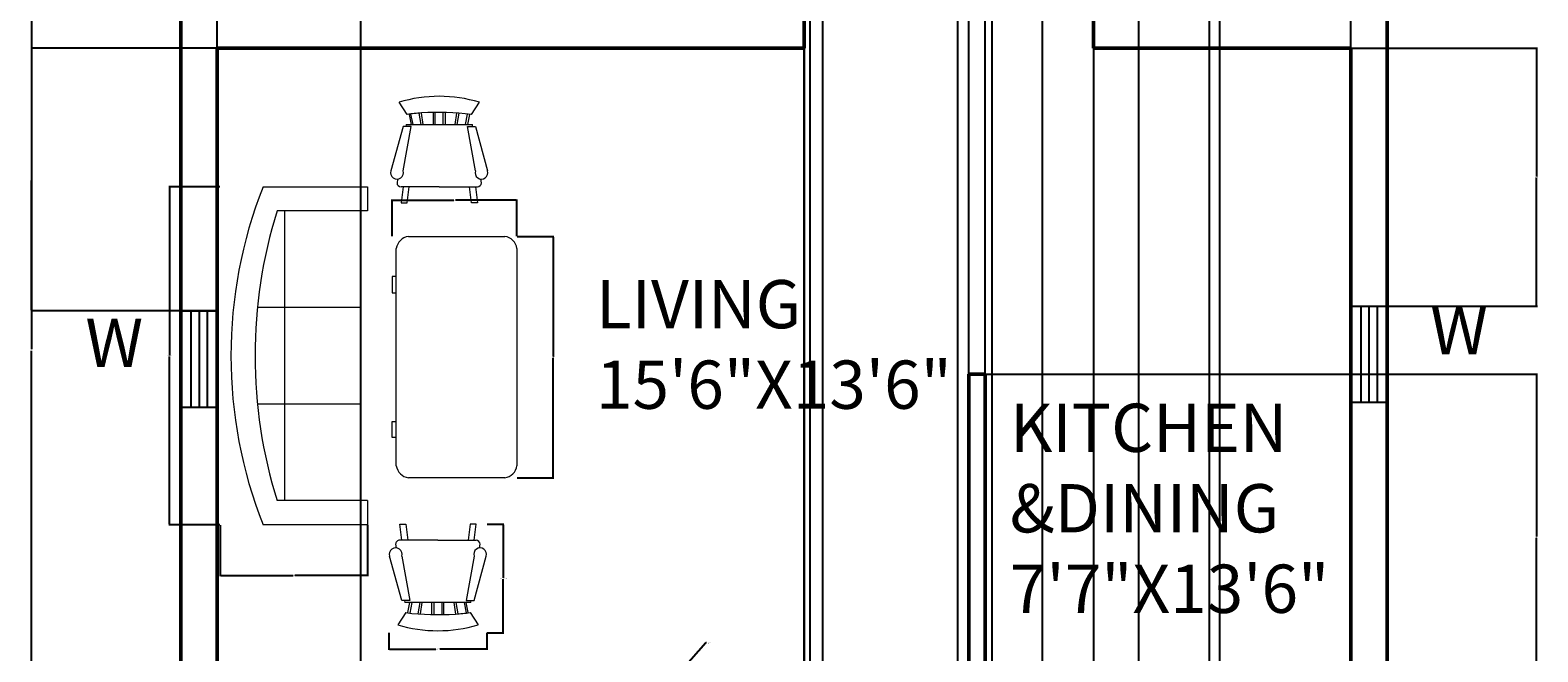
# Model space of a CAD drawing. Units: inches. Extents: x -15 to 361, y -684 to 58.
# Tile 2 of 3: x -15 to 360, y -385 to -230. Entities that reach past the tile are written whole.
import ezdxf

# ---------------------------------------------------------------- set-up
doc = ezdxf.new("R2010")
doc.units = ezdxf.units.IN
doc.header["$MEASUREMENT"] = 0
for name, color, linetype, lineweight in [('A-ANNO-DIMS', 2, 'Continuous', 18), ('A-ANNO-TEXT', 7, 'Continuous', 18), ('A-AREA-IDEN', 7, 'Continuous', 25), ('A-FURN', 8, 'Continuous', 18), ('A-GLAZ', 4, 'Continuous', 25), ('A-WALL', 7, 'Continuous', 50)]:
    doc.layers.add(name, color=color, linetype=linetype, lineweight=lineweight)
doc.styles.get("Standard").update_dxf_attribs({"font": 'arial.ttf'})
doc.dimstyles.get("Standard").update_dxf_attribs({"dimtxt": 0.18, "dimasz": 0.18, "dimexe": 0.18, "dimexo": 0.0625, "dimgap": 0.09, "dimtad": 0, "dimtih": 1, "dimtoh": 1, "dimdec": 4, "dimzin": 0, "dimdsep": 46, "dimtxsty": 'Standard', "dimcen": 0.09, "dimadec": 0, "dimazin": 0, "dimtfac": 1, "dimtdec": 4, "dimtofl": 0, "dimtmove": 0, "dimatfit": 3, "dimfxl": 1, "dimtolj": 1, "dimtzin": 0, "dimarcsym": 0})

# ---------------------------------------------------------------- blocks, each defined once
blk = doc.blocks.new('Chair - Rocking')
for p, q in [((-8, -4.5), (-10, -1.5)), ((8, -4.5), (10, -1.5)), ((-9, -7.5), (-12, -18.49999)), ((-7, -7.5), (-9, -7.5)), ((-9, -18.49999), (-7, -7.5)), ((-8.23428, -6.99939), (-8.3093, -7.47958)), ((-8.23041, -7), (8.23915, -7)), ((-7.5, -4.5), (-7, -7)), ((-6.5, -7), (-7.02225, -4.43)), ((-4.5, -7), (-4.96674, -4.19951)), ((-4, -7), (-4.40532, -4.16272)), ((-1.5, -4.05012), (-1.5, -7)), ((-1, -7), (-1, -4.05012)), ((1, -7), (1, -4.04655)), ((1.5, -4.05012), (1.5, -7)), ((4, -7), (4.40187, -4.18694)), ((4.5, -7), (4.96761, -4.19437)), ((6.5, -7), (7, -4.4057)), ((7.5, -4.5), (7, -7)), ((7, -7.5), (9, -7.5)), ((9, -18.49999), (7, -7.5)), ((8.31071, -7.48854), (8.23449, -7.00073)), ((9, -7.5), (12, -18.49999)), ((-10.36644, -20.64523), (-10.5, -21.49999)), ((-9, -22.49999), (-9.5, -26.49999)), ((0, -22.49999), (-9.5, -22.49999)), ((-8, -26.49999), (-7.5, -22.49999)), ((0, -22.49999), (9.5, -22.49999)), ((8, -26.49999), (7.5, -22.49999)), ((9, -22.49999), (9.5, -26.49999)), ((10.5, -21.49999), (10.3575, -20.58798)), ((-9.5, -26.49999), (-8, -26.49999)), ((9.5, -26.49999), (8, -26.49999))]:
    blk.add_line(p, q)
for centre, radius, start, end in [((0, -34.08333), 34.08333, 72.93847, 107.0615), ((0, -68.25004), 64.25, 93.92211, 97.15267), ((0, -68.25004), 64.25, 82.84733, 93.92211), ((-10.5, -18.99999), 1.58114, 161.5651, 18.43495), ((10.5, -18.99999), 1.58114, 161.5651, 18.43495), ((-9.5, -21.49999), 1, 180, 270), ((9.5, -21.49999), 1, 270, 0)]:
    blk.add_arc(centre, radius, start, end)
blk = doc.blocks.new('Sofa - Roundback 7 ft.')
for p, q in [((-12.00002, -32.4421), (-12.00003, -6.5971)), ((11.99997, -32.4421), (11.99998, -6.5971)), ((-36.000027, -34), (-36.000027, -11.4696)), ((-35.999844, -13.3819), (35.9998, -13.3819)), ((35.99998, -34), (35.99998, -11.4696)), ((-36.000027, -32.4421), (35.99998, -32.4421))]:
    blk.add_line(p, q)
for points in [[(-36.000027, -34), (-42.000027, -34), (-42.000027, -8)], [(41.99998, -8), (41.99998, -34), (35.99998, -34)]]:
    blk.add_lwpolyline(points)
for centre, radius, start, end in [((0, -114.25), 114.25, 68.43141, 111.5686), ((-0.00001, -127.1968), 121.1968, 72.72033, 107.2797)]:
    blk.add_arc(centre, radius, start, end)
blk = doc.blocks.new('Desk - 30 x 60 in.')
for p, q in [((-26.999995, 0), (26.999995, 0)), ((-29.999995, -27), (-29.999995, -3)), ((29.999995, -3), (29.999995, -27)), ((26.999995, -30), (-26.999995, -30)), ((-20.000005, -30), (-20.000005, -31)), ((-16.000005, -31), (-16.000005, -30)), ((15.999995, -31), (15.999995, -30)), ((19.999995, -30), (19.999995, -31)), ((-20.000005, -31), (-16.000005, -31)), ((19.999995, -31), (15.999995, -31))]:
    blk.add_line(p, q)
for centre, start, end in [((-26.499995, -3.5), 98.1301, 171.8699), ((26.499995, -3.5), 8.130102, 81.8699), ((-26.499995, -26.5), 188.1301, 261.8699), ((26.499995, -26.5), 278.1301, 351.8699)]:
    blk.add_arc(centre, 3.535534, start, end)
blk = doc.blocks.new('WIN-24IN')
for p, q in [((0, 6.5), (24, 6.5)), ((0, 4.5), (24, 4.5)), ((0, 2.5), (24, 2.5))]:
    blk.add_line(p, q)
blk.add_lwpolyline([(0, 9), (24, 9), (24, 0), (0, 0)], close=True)
blk = doc.blocks.new('*D15')
at = {"layer": 'A-ANNO-DIMS', "color": 0, "lineweight": -2, "transparency": 16777216}
for p, q in [((99.11, -352.97), (103.28, -352.97)), ((103.1, -353.15), (103.1, -366.29)), ((103.1, -379.79), (103.1, -366.66)), ((99.11, -379.97), (103.28, -379.97))]:
    blk.add_line(p, q, dxfattribs=at)
at = {"layer": 'A-ANNO-DIMS', "color": 0, "transparency": 16777216}
for points in [[(103.07, -353.15), (103.13, -353.15), (103.1, -352.97)], [(103.07, -379.79), (103.13, -379.79), (103.1, -379.97)]]:
    blk.add_solid(points, dxfattribs=at)
at = {"layer": 'Defpoints', "color": 0, "transparency": 16777216}
for p in [(99.05, -352.97), (99.05, -379.97), (103.1, -379.97)]:
    blk.add_point(p, dxfattribs=at)
at = {"layer": 'A-ANNO-DIMS', "color": 0, "transparency": 16777216, "insert": (103.1, -366.47), "char_height": 0.18, "attachment_point": 5}
blk.add_mtext('\\A1;ROCKER 27 TYP.', dxfattribs=at)
blk = doc.blocks.new('*D16')
at = {"layer": 'A-ANNO-DIMS', "color": 0, "lineweight": -2, "transparency": 16777216}
for p, q in [((74.62, -380.03), (74.62, -384.2)), ((99.05, -380.03), (99.05, -384.2)), ((74.8, -384.02), (86.3, -384.02)), ((98.87, -384.02), (87.36, -384.02))]:
    blk.add_line(p, q, dxfattribs=at)
at = {"layer": 'A-ANNO-DIMS', "color": 0, "transparency": 16777216}
for points in [[(74.8, -383.99), (74.8, -384.05), (74.62, -384.02)], [(98.87, -383.99), (98.87, -384.05), (99.05, -384.02)]]:
    blk.add_solid(points, dxfattribs=at)
at = {"layer": 'Defpoints', "color": 0, "transparency": 16777216}
for p in [(74.62, -379.97), (99.05, -379.97), (74.62, -384.02)]:
    blk.add_point(p, dxfattribs=at)
at = {"layer": 'A-ANNO-DIMS', "color": 0, "transparency": 16777216, "insert": (86.83, -384.02), "char_height": 0.18, "attachment_point": 5}
blk.add_mtext('\\A1;24 TYP.', dxfattribs=at)
blk = doc.blocks.new('*D17')
at = {"layer": 'A-ANNO-DIMS', "color": 0, "lineweight": -2, "transparency": 16777216}
for p, q in [((32.62, -269.13), (19.91, -269.13)), ((20.09, -269.31), (20.09, -310.94)), ((20.09, -352.95), (20.09, -311.31)), ((32.62, -353.13), (19.91, -353.13))]:
    blk.add_line(p, q, dxfattribs=at)
at = {"layer": 'A-ANNO-DIMS', "color": 0, "transparency": 16777216}
for points in [[(20.06, -269.31), (20.12, -269.31), (20.09, -269.13)], [(20.06, -352.95), (20.12, -352.95), (20.09, -353.13)]]:
    blk.add_solid(points, dxfattribs=at)
at = {"layer": 'Defpoints', "color": 0, "transparency": 16777216}
for p in [(20.09, -269.13), (32.69, -269.13), (32.69, -353.13)]:
    blk.add_point(p, dxfattribs=at)
at = {"layer": 'A-ANNO-DIMS', "color": 0, "transparency": 16777216, "insert": (20.09, -311.13), "char_height": 0.18, "attachment_point": 5}
blk.add_mtext('\\A1;SOFA 84', dxfattribs=at)
blk = doc.blocks.new('*D18')
at = {"layer": 'A-ANNO-DIMS', "color": 0, "lineweight": -2, "transparency": 16777216}
for p, q in [((32.69, -353.19), (32.69, -365.91)), ((69.35, -353.19), (69.35, -365.91)), ((32.87, -365.73), (50.8, -365.73)), ((69.17, -365.73), (51.24, -365.73))]:
    blk.add_line(p, q, dxfattribs=at)
at = {"layer": 'A-ANNO-DIMS', "color": 0, "transparency": 16777216}
for points in [[(32.87, -365.7), (32.87, -365.76), (32.69, -365.73)], [(69.17, -365.7), (69.17, -365.76), (69.35, -365.73)]]:
    blk.add_solid(points, dxfattribs=at)
at = {"layer": 'Defpoints', "color": 0, "transparency": 16777216}
for p in [(32.69, -353.13), (69.35, -353.13), (32.69, -365.73)]:
    blk.add_point(p, dxfattribs=at)
at = {"layer": 'A-ANNO-DIMS', "color": 0, "transparency": 16777216, "insert": (51.02, -365.73), "char_height": 0.18, "attachment_point": 5}
blk.add_mtext('\\A1;37', dxfattribs=at)
blk = doc.blocks.new('*D19')
at = {"layer": 'A-ANNO-DIMS', "color": 0, "lineweight": -2, "transparency": 16777216}
for p, q in [((106.56, -281.45), (115.68, -281.45)), ((115.5, -281.63), (115.5, -311.27)), ((115.5, -341.27), (115.5, -311.63)), ((106.56, -341.45), (115.68, -341.45))]:
    blk.add_line(p, q, dxfattribs=at)
at = {"layer": 'A-ANNO-DIMS', "color": 0, "transparency": 16777216}
for points in [[(115.47, -281.63), (115.53, -281.63), (115.5, -281.45)], [(115.47, -341.27), (115.53, -341.27), (115.5, -341.45)]]:
    blk.add_solid(points, dxfattribs=at)
at = {"layer": 'Defpoints', "color": 0, "transparency": 16777216}
for p in [(106.5, -281.45), (106.5, -341.45), (115.5, -341.45)]:
    blk.add_point(p, dxfattribs=at)
at = {"layer": 'A-ANNO-DIMS', "color": 0, "transparency": 16777216, "insert": (115.5, -311.45), "char_height": 0.18, "attachment_point": 5}
blk.add_mtext('\\A1;DESK 60', dxfattribs=at)
blk = doc.blocks.new('*D20')
at = {"layer": 'A-ANNO-DIMS', "color": 0, "lineweight": -2, "transparency": 16777216}
for p, q in [((75.5, -281.39), (75.5, -272.27)), ((75.68, -272.45), (90.8, -272.45)), ((106.32, -272.45), (91.2, -272.45)), ((106.5, -281.39), (106.5, -272.27))]:
    blk.add_line(p, q, dxfattribs=at)
at = {"layer": 'A-ANNO-DIMS', "color": 0, "transparency": 16777216}
for points in [[(75.68, -272.42), (75.68, -272.48), (75.5, -272.45)], [(106.32, -272.42), (106.32, -272.48), (106.5, -272.45)]]:
    blk.add_solid(points, dxfattribs=at)
at = {"layer": 'Defpoints', "color": 0, "transparency": 16777216}
for p in [(106.5, -272.45), (75.5, -281.45), (106.5, -281.45)]:
    blk.add_point(p, dxfattribs=at)
at = {"layer": 'A-ANNO-DIMS', "color": 0, "transparency": 16777216, "insert": (91, -272.45), "char_height": 0.18, "attachment_point": 5}
blk.add_mtext('\\A1;31', dxfattribs=at)
blk = doc.blocks.new('*D24')
at = {"layer": 'A-ANNO-DIMS', "color": 0, "lineweight": -2, "transparency": 16777216}
for p, q in [((22.87, 20.31), (-14.45, 20.31)), ((-14.27, 20.13), (-14.27, -309.51)), ((-14.27, -639.51), (-14.27, -309.87)), ((22.87, -639.69), (-14.45, -639.69))]:
    blk.add_line(p, q, dxfattribs=at)
at = {"layer": 'A-ANNO-DIMS', "color": 0, "transparency": 16777216}
for points in [[(-14.3, 20.13), (-14.24, 20.13), (-14.27, 20.31)], [(-14.3, -639.51), (-14.24, -639.51), (-14.27, -639.69)]]:
    blk.add_solid(points, dxfattribs=at)
at = {"layer": 'Defpoints', "color": 0, "transparency": 16777216}
for p in [(-14.27, 20.31), (22.93, 20.31), (22.93, -639.69)]:
    blk.add_point(p, dxfattribs=at)
at = {"layer": 'A-ANNO-DIMS', "color": 0, "transparency": 16777216, "insert": (-14.27, -309.69), "char_height": 0.18, "attachment_point": 5}
blk.add_mtext('\\A1;660', dxfattribs=at)
blk = doc.blocks.new('*D28')
at = {"layer": 'A-ANNO-DIMS', "color": 0, "lineweight": -2, "transparency": 16777216}
for p, q in [((313.99, -234.69), (360.31, -234.69)), ((360.13, -234.87), (360.13, -266.55)), ((360.13, -298.6), (360.13, -266.92)), ((313.99, -298.78), (360.31, -298.78))]:
    blk.add_line(p, q, dxfattribs=at)
at = {"layer": 'A-ANNO-DIMS', "color": 0, "transparency": 16777216}
for points in [[(360.1, -234.87), (360.16, -234.87), (360.13, -234.69)], [(360.1, -298.6), (360.16, -298.6), (360.13, -298.78)]]:
    blk.add_solid(points, dxfattribs=at)
at = {"layer": 'Defpoints', "color": 0, "transparency": 16777216}
for p in [(313.93, -234.69), (313.93, -298.78), (360.13, -298.78)]:
    blk.add_point(p, dxfattribs=at)
at = {"layer": 'A-ANNO-DIMS', "color": 0, "transparency": 16777216, "insert": (360.13, -266.73), "char_height": 0.18, "attachment_point": 5}
blk.add_mtext('\\A1;64.08', dxfattribs=at)
blk = doc.blocks.new('*D31')
at = {"layer": 'A-ANNO-DIMS', "color": 0, "lineweight": -2, "transparency": 16777216}
for p, q in [((177.93, -549.63), (177.93, 57.69)), ((178.11, 57.51), (207.18, 57.51)), ((237.04, 57.51), (207.97, 57.51)), ((237.22, -549.63), (237.22, 57.69))]:
    blk.add_line(p, q, dxfattribs=at)
at = {"layer": 'A-ANNO-DIMS', "color": 0, "transparency": 16777216}
for points in [[(178.11, 57.54), (178.11, 57.48), (177.93, 57.51)], [(237.04, 57.54), (237.04, 57.48), (237.22, 57.51)]]:
    blk.add_solid(points, dxfattribs=at)
at = {"layer": 'Defpoints', "color": 0, "transparency": 16777216}
for p in [(237.22, 57.51), (177.93, -549.69), (237.22, -549.69)]:
    blk.add_point(p, dxfattribs=at)
at = {"layer": 'A-ANNO-DIMS', "color": 0, "transparency": 16777216, "insert": (207.57, 57.51), "char_height": 0.18, "attachment_point": 5}
blk.add_mtext('\\A1;59.29', dxfattribs=at)
blk = doc.blocks.new('*D32')
at = {"layer": 'A-ANNO-DIMS', "color": 0, "lineweight": -2, "transparency": 16777216}
for p, q in [((31.93, -396.63), (31.93, 57.69)), ((32.11, 57.51), (49.42, 57.51)), ((67.52, 57.51), (50.21, 57.51)), ((67.7, -396.63), (67.7, 57.69))]:
    blk.add_line(p, q, dxfattribs=at)
at = {"layer": 'A-ANNO-DIMS', "color": 0, "transparency": 16777216}
for points in [[(32.11, 57.54), (32.11, 57.48), (31.93, 57.51)], [(67.52, 57.54), (67.52, 57.48), (67.7, 57.51)]]:
    blk.add_solid(points, dxfattribs=at)
at = {"layer": 'Defpoints', "color": 0, "transparency": 16777216}
for p in [(67.7, 57.51), (31.93, -396.69), (67.7, -396.69)]:
    blk.add_point(p, dxfattribs=at)
at = {"layer": 'A-ANNO-DIMS', "color": 0, "transparency": 16777216, "insert": (49.81, 57.51), "char_height": 0.18, "attachment_point": 5}
blk.add_mtext('\\A1;35.77', dxfattribs=at)
blk = doc.blocks.new('*D34')
at = {"layer": 'A-ANNO-DIMS', "color": 0, "lineweight": -2, "transparency": 16777216}
for p, q in [((31.87, -234.69), (-14.45, -234.69)), ((-14.27, -234.87), (-14.27, -267.15)), ((-14.27, -299.8), (-14.27, -267.52)), ((31.87, -299.98), (-14.45, -299.98))]:
    blk.add_line(p, q, dxfattribs=at)
at = {"layer": 'A-ANNO-DIMS', "color": 0, "transparency": 16777216}
for points in [[(-14.3, -234.87), (-14.24, -234.87), (-14.27, -234.69)], [(-14.3, -299.8), (-14.24, -299.8), (-14.27, -299.98)]]:
    blk.add_solid(points, dxfattribs=at)
at = {"layer": 'Defpoints', "color": 0, "transparency": 16777216}
for p in [(31.93, -234.69), (-14.27, -299.98), (31.93, -299.98)]:
    blk.add_point(p, dxfattribs=at)
at = {"layer": 'A-ANNO-DIMS', "color": 0, "transparency": 16777216, "insert": (-14.27, -267.34), "char_height": 0.18, "attachment_point": 5}
blk.add_mtext('\\A1;65.29', dxfattribs=at)
blk = doc.blocks.new('*D37')
at = {"layer": 'A-ANNO-DIMS', "color": 0, "lineweight": -2, "transparency": 16777216}
for p, q in [((182.53, -153.75), (182.53, -677.07)), ((224.64, -153.75), (224.64, -677.07)), ((182.71, -676.89), (203.21, -676.89)), ((224.46, -676.89), (203.97, -676.89))]:
    blk.add_line(p, q, dxfattribs=at)
at = {"layer": 'A-ANNO-DIMS', "color": 0, "transparency": 16777216}
for points in [[(182.71, -676.86), (182.71, -676.92), (182.53, -676.89)], [(224.46, -676.86), (224.46, -676.92), (224.64, -676.89)]]:
    blk.add_solid(points, dxfattribs=at)
at = {"layer": 'Defpoints', "color": 0, "transparency": 16777216}
for p in [(182.53, -153.69), (224.64, -153.69), (224.64, -676.89)]:
    blk.add_point(p, dxfattribs=at)
at = {"layer": 'A-ANNO-DIMS', "color": 0, "transparency": 16777216, "insert": (203.59, -676.89), "char_height": 0.18, "attachment_point": 5}
blk.add_mtext('\\A1;42.11', dxfattribs=at)
blk = doc.blocks.new('*D42')
at = {"layer": 'A-ANNO-DIMS', "color": 0, "lineweight": -2, "transparency": 16777216}
for p, q in [((179.42, -396.63), (179.42, 57.69)), ((179.6, 57.51), (197.42, 57.51)), ((216.02, 57.51), (198.21, 57.51)), ((216.2, -396.63), (216.2, 57.69))]:
    blk.add_line(p, q, dxfattribs=at)
at = {"layer": 'A-ANNO-DIMS', "color": 0, "transparency": 16777216}
for points in [[(179.6, 57.54), (179.6, 57.48), (179.42, 57.51)], [(216.02, 57.54), (216.02, 57.48), (216.2, 57.51)]]:
    blk.add_solid(points, dxfattribs=at)
at = {"layer": 'Defpoints', "color": 0, "transparency": 16777216}
for p in [(216.2, 57.51), (179.42, -396.69), (216.2, -396.69)]:
    blk.add_point(p, dxfattribs=at)
at = {"layer": 'A-ANNO-DIMS', "color": 0, "transparency": 16777216, "insert": (197.81, 57.51), "char_height": 0.18, "attachment_point": 5}
blk.add_mtext('\\A1;36.78', dxfattribs=at)
blk = doc.blocks.new('*D44')
at = {"layer": 'A-ANNO-DIMS', "color": 0, "lineweight": -2, "transparency": 16777216}
for p, q in [((281.35, -558.63), (281.35, 57.69)), ((281.53, 57.51), (297.18, 57.51)), ((313.75, 57.51), (298.1, 57.51)), ((313.93, -558.63), (313.93, 57.69))]:
    blk.add_line(p, q, dxfattribs=at)
at = {"layer": 'A-ANNO-DIMS', "color": 0, "transparency": 16777216}
for points in [[(281.53, 57.54), (281.53, 57.48), (281.35, 57.51)], [(313.75, 57.54), (313.75, 57.48), (313.93, 57.51)]]:
    blk.add_solid(points, dxfattribs=at)
at = {"layer": 'Defpoints', "color": 0, "transparency": 16777216}
for p in [(313.93, 57.51), (281.35, -558.69), (313.93, -558.69)]:
    blk.add_point(p, dxfattribs=at)
at = {"layer": 'A-ANNO-DIMS', "color": 0, "transparency": 16777216, "insert": (297.64, 57.51), "char_height": 0.18, "attachment_point": 5}
blk.add_mtext('\\A1;32.575', dxfattribs=at)
blk = doc.blocks.new('*D48')
at = {"layer": 'A-ANNO-DIMS', "color": 0, "lineweight": -2, "transparency": 16777216}
for p, q in [((222.99, -315.69), (360.31, -315.69)), ((360.13, -315.87), (360.13, -356.01)), ((360.13, -396.51), (360.13, -356.37)), ((222.99, -396.69), (360.31, -396.69))]:
    blk.add_line(p, q, dxfattribs=at)
at = {"layer": 'A-ANNO-DIMS', "color": 0, "transparency": 16777216}
for points in [[(360.1, -315.87), (360.16, -315.87), (360.13, -315.69)], [(360.1, -396.51), (360.16, -396.51), (360.13, -396.69)]]:
    blk.add_solid(points, dxfattribs=at)
at = {"layer": 'Defpoints', "color": 0, "transparency": 16777216}
for p in [(222.93, -315.69), (360.13, -315.69), (222.93, -396.69)]:
    blk.add_point(p, dxfattribs=at)
at = {"layer": 'A-ANNO-DIMS', "color": 0, "transparency": 16777216, "insert": (360.13, -356.19), "char_height": 0.18, "attachment_point": 5}
blk.add_mtext('\\A1;81', dxfattribs=at)
blk = doc.blocks.new('*D49')
at = {"layer": 'A-ANNO-DIMS', "color": 0, "lineweight": -2, "transparency": 16777216}
for p, q in [((218.93, -315.63), (218.93, 57.69)), ((219.11, 57.51), (220.78, 57.51)), ((222.75, 57.51), (221.08, 57.51)), ((222.93, -315.63), (222.93, 57.69))]:
    blk.add_line(p, q, dxfattribs=at)
at = {"layer": 'A-ANNO-DIMS', "color": 0, "transparency": 16777216}
for points in [[(219.11, 57.54), (219.11, 57.48), (218.93, 57.51)], [(222.75, 57.54), (222.75, 57.48), (222.93, 57.51)]]:
    blk.add_solid(points, dxfattribs=at)
at = {"layer": 'Defpoints', "color": 0, "transparency": 16777216}
for p in [(222.93, 57.51), (218.93, -315.69), (222.93, -315.69)]:
    blk.add_point(p, dxfattribs=at)
at = {"layer": 'A-ANNO-DIMS', "color": 0, "transparency": 16777216, "insert": (220.93, 57.51), "char_height": 0.18, "attachment_point": 5}
blk.add_mtext('\\A1;4', dxfattribs=at)
blk = doc.blocks.new('*D50')
at = {"layer": 'A-ANNO-DIMS', "color": 0, "lineweight": -2, "transparency": 16777216}
for p, q in [((177.93, -234.75), (177.93, -677.07)), ((249.93, -234.75), (249.93, -677.07)), ((178.11, -676.89), (213.71, -676.89)), ((249.75, -676.89), (214.15, -676.89))]:
    blk.add_line(p, q, dxfattribs=at)
at = {"layer": 'A-ANNO-DIMS', "color": 0, "transparency": 16777216}
for points in [[(178.11, -676.86), (178.11, -676.92), (177.93, -676.89)], [(249.75, -676.86), (249.75, -676.92), (249.93, -676.89)]]:
    blk.add_solid(points, dxfattribs=at)
at = {"layer": 'Defpoints', "color": 0, "transparency": 16777216}
for p in [(177.93, -234.69), (249.93, -234.69), (249.93, -676.89)]:
    blk.add_point(p, dxfattribs=at)
at = {"layer": 'A-ANNO-DIMS', "color": 0, "transparency": 16777216, "insert": (213.93, -676.89), "char_height": 0.18, "attachment_point": 5}
blk.add_mtext('\\A1;72', dxfattribs=at)
blk = doc.blocks.new('*D52')
at = {"layer": 'A-ANNO-DIMS', "color": 0, "lineweight": -2, "transparency": 16777216}
for p, q in [((261.22, -549.63), (261.22, 57.69)), ((261.4, 57.51), (269.54, 57.51)), ((278.6, 57.51), (270.45, 57.51)), ((278.78, -549.63), (278.78, 57.69))]:
    blk.add_line(p, q, dxfattribs=at)
at = {"layer": 'A-ANNO-DIMS', "color": 0, "transparency": 16777216}
for points in [[(261.4, 57.54), (261.4, 57.48), (261.22, 57.51)], [(278.6, 57.54), (278.6, 57.48), (278.78, 57.51)]]:
    blk.add_solid(points, dxfattribs=at)
at = {"layer": 'Defpoints', "color": 0, "transparency": 16777216}
for p in [(278.78, 57.51), (261.22, -549.69), (278.78, -549.69)]:
    blk.add_point(p, dxfattribs=at)
at = {"layer": 'A-ANNO-DIMS', "color": 0, "transparency": 16777216, "insert": (270, 57.51), "char_height": 0.18, "attachment_point": 5}
blk.add_mtext('\\A1;17.564', dxfattribs=at)
blk = doc.blocks.new('*D58')
at = {"layer": 'A-ANNO-DIMS', "color": 0, "lineweight": -2, "transparency": 16777216}
for p, q in [((153.48, -382.49), (144.4, -392.86)), ((153.66, -382.49), (153.48, -382.49)), ((128.87, -410.51), (129.05, -410.51)), ((128.96, -410.6), (128.96, -410.42))]:
    blk.add_line(p, q, dxfattribs=at)
at = {"layer": 'A-ANNO-DIMS', "color": 0, "transparency": 16777216}
blk.add_solid([(144.38, -392.84), (144.42, -392.88), (144.28, -393)], dxfattribs=at)
at = {"layer": 'Defpoints', "color": 0, "transparency": 16777216}
for p in [(144.28, -393), (128.96, -410.51)]:
    blk.add_point(p, dxfattribs=at)
at = {"layer": 'A-ANNO-DIMS', "color": 0, "transparency": 16777216, "insert": (154.21, -382.49), "char_height": 0.18, "attachment_point": 5}
blk.add_mtext('\\A1;R23.274', dxfattribs=at)

msp = doc.modelspace()

# ---------------------------------------------------------------- linework, layer by layer
at = {"layer": 'A-WALL'}
for p, q in [((249.9279, -223.2006), (249.9279, -234.6922)), ((177.9279, -225.6922), (177.9279, -234.6922)), ((31.9279, -234.6922), (177.9279, -234.6922)), ((31.9279, -396.6922), (31.9279, -234.6922)), ((249.9279, -234.6922), (313.9279, -234.6922)), ((313.9279, -234.6922), (313.9279, -396.6922)), ((218.9279, -315.6922), (222.9279, -315.6922)), ((218.9279, -315.6922), (218.9279, -396.6922)), ((222.9279, -315.6922), (222.9279, -396.6922))]:
    msp.add_line(p, q, dxfattribs=at)
msp.add_lwpolyline([(31.9279, -639.6922), (22.9279, -639.6922), (22.9279, 20.3078), (322.9279, 20.3078), (322.9279, -639.6922), (137.4946, -639.6922)], dxfattribs=at)

# ---------------------------------------------------------------- block references
at = {"layer": 'A-FURN'}
msp.add_blockref('Chair - Rocking', (87.1719, -246.626), dxfattribs=at)
for name, p, rotation in [('Sofa - Roundback 7 ft.', (35.3525, -311.1259), 89.99995792911221), ('Desk - 30 x 60 in.', (106.5013, -311.4492), 270), ('Chair - Rocking', (86.8342, -379.4722), 180)]:
    msp.add_blockref(name, p, dxfattribs=dict(at, rotation=rotation))
at = {"layer": 'A-GLAZ', "rotation": 270.0000000000002}
for p in [(22.9281, -299.9803), (313.9281, -298.7754)]:
    msp.add_blockref('WIN-24IN', p, dxfattribs=at)

# ---------------------------------------------------------------- texts
at = {"layer": 'A-ANNO-TEXT', "char_height": 12, "attachment_point": 1}
for width, insert in [(36.724231, (333.6435, -298.7757)), (23.776044, (-0.8482, -301.8853))]:
    msp.add_mtext_dynamic_manual_height_columns('W', width=width, gutter_width=60, heights=[0], dxfattribs=dict(at, insert=insert))
at = {"layer": 'A-AREA-IDEN', "char_height": 12, "attachment_point": 1}
for s, width, insert in [('LIVING\\P15\'6"X13\'6"', 66.743833, (126.1571, -292.2987)), ('KITCHEN\\P&DINING\\P7\'7"X13\'6"', 78.770856, (229.1231, -323.0223))]:
    msp.add_mtext_dynamic_manual_height_columns(s, width=width, gutter_width=60, heights=[0], dxfattribs=dict(at, insert=insert))

# ---------------------------------------------------------------- dimensions: what is measured, and where the dimension line sits
at = {"layer": 'A-ANNO-DIMS'}
for base, p1, p2, override, picture, middle in [((67.6973, 57.5078), (31.9279, -396.6922), (67.6973, -396.6922), {"dimdec": 2, "dimlfac": 1, "dimrnd": 0, "dimzin": 0, "dimdsep": 46, "dimlunit": 2}, '*D32', (49.8126, 57.5078)), ((237.2164, 57.5078), (177.9279, -549.6922), (237.2164, -549.6922), {"dimdec": 2, "dimlfac": 1, "dimrnd": 0, "dimzin": 0, "dimdsep": 46, "dimlunit": 2}, '*D31', (207.5721, 57.5078)), ((216.2043, 57.5078), (179.4234, -396.6922), (216.2043, -396.6922), {"dimdec": 2, "dimlfac": 1, "dimrnd": 0, "dimzin": 0, "dimdsep": 46, "dimlunit": 2}, '*D42', (197.8139, 57.5078)), ((222.9279, 57.5078), (218.9279, -315.6922), (222.9279, -315.6922), {"dimdec": 0, "dimlfac": 1, "dimrnd": 0, "dimzin": 0, "dimdsep": 46, "dimlunit": 2}, '*D49', (220.9279, 57.5078)), ((278.78086, 57.50778), (261.21639, -549.69222), (278.78086, -549.69222), {"dimdec": 3, "dimlfac": 1, "dimrnd": 0, "dimzin": 0, "dimdsep": 46, "dimlunit": 2}, '*D52', (269.99863, 57.50778)), ((313.9279, 57.5078), (281.3528, -558.6922), (313.9279, -558.6922), {"dimdec": 3, "dimlfac": 1, "dimrnd": 0, "dimzin": 0, "dimdsep": 46, "dimlunit": 2}, '*D44', (297.6403, 57.5078)), ((224.6415, -676.8922), (182.5334, -153.6922), (224.6415, -153.6922), {"dimdec": 2, "dimlfac": 1, "dimrnd": 0, "dimzin": 0, "dimdsep": 46, "dimlunit": 2}, '*D37', (203.5874, -676.8922)), ((249.9279, -676.8922), (177.9279, -234.6922), (249.9279, -234.6922), {"dimdec": 0, "dimlfac": 1, "dimrnd": 0, "dimzin": 0, "dimdsep": 46, "dimlunit": 2}, '*D50', (213.9279, -676.8922)), ((106.5013, -272.4492), (75.5013, -281.4492), (106.5013, -281.4492), {"dimdec": 0, "dimlfac": 1, "dimrnd": 0, "dimzin": 0, "dimdsep": 46, "dimlunit": 2}, '*D20', (91.0013, -272.4492))]:
    dim = msp.add_linear_dim(base=base, p1=p1, p2=p2, dimstyle='Standard', override=override, dxfattribs=at)
    dim.commit()
    dim.dimension.update_dxf_attribs({"geometry": picture, "text_midpoint": middle})
for base, p1, p2, angle, override, picture, middle in [((-14.2721, 20.3078), (22.9279, -639.6922), (22.9279, 20.3078), 90, {"dimdec": 0, "dimlfac": 1, "dimrnd": 0, "dimzin": 0, "dimdsep": 46, "dimlunit": 2}, '*D24', (-14.2721, -309.6922)), ((-14.2721, -299.9807), (31.9279, -234.6922), (31.9279, -299.9807), 90, {"dimdec": 2, "dimlfac": 1, "dimrnd": 0, "dimzin": 0, "dimdsep": 46, "dimlunit": 2}, '*D34', (-14.2721, -267.3365)), ((360.1279, -298.7757), (313.9279, -234.6922), (313.9279, -298.7757), 90, {"dimdec": 2, "dimlfac": 1, "dimrnd": 0, "dimzin": 0, "dimdsep": 46, "dimlunit": 2}, '*D28', (360.1279, -266.734)), ((360.1279, -315.6922), (222.9279, -396.6922), (222.9279, -315.6922), 90, {"dimdec": 0, "dimlfac": 1, "dimrnd": 0, "dimzin": 0, "dimdsep": 46, "dimlunit": 2}, '*D48', (360.1279, -356.1922)), ((32.6857, -365.726), (69.3524, -353.126), (32.6858, -353.126), 179.999958, {"dimdec": 0, "dimlfac": 1, "dimrnd": 0, "dimzin": 0, "dimdsep": 46, "dimlunit": 2}, '*D18', (51.0191, -365.726))]:
    dim = msp.add_linear_dim(base=base, p1=p1, p2=p2, angle=angle, dimstyle='Standard', override=override, dxfattribs=at)
    dim.commit()
    dim.dimension.update_dxf_attribs({"geometry": picture, "text_midpoint": middle})
for base, p1, p2, angle, text, picture, middle in [((20.0858, -269.1259), (32.6858, -353.126), (32.6858, -269.1259), 89.999958, 'SOFA <>', '*D17', (20.0858, -311.126)), ((115.5012, -341.4492), (106.5013, -281.4492), (106.5013, -341.4492), 270, 'DESK <>', '*D19', (115.5012, -311.4492)), ((103.1017, -379.9722), (99.0517, -352.9722), (99.0517, -379.9722), 270, 'ROCKER <> TYP.', '*D15', (103.1017, -366.4722)), ((74.6166, -384.0222), (99.0517, -379.9722), (74.6166, -379.9722), 180, '<> TYP.', '*D16', (86.8342, -384.0222))]:
    dim = msp.add_linear_dim(base=base, p1=p1, p2=p2, angle=angle, text=text, dimstyle='Standard', override={"dimdec": 0, "dimlfac": 1, "dimrnd": 0, "dimzin": 0, "dimdsep": 46, "dimlunit": 2}, dxfattribs=at)
    dim.commit()
    dim.dimension.update_dxf_attribs({"geometry": picture, "text_midpoint": middle})
dim = msp.add_radius_dim(center=(128.958, -410.5149), mpoint=(144.283, -392.999), dimstyle='Standard', override={"dimdec": 3, "dimlfac": 1, "dimrnd": 0, "dimzin": 0, "dimdsep": 46, "dimlunit": 2}, dxfattribs=at)
dim.commit()
dim.dimension.update_dxf_attribs({"geometry": '*D58', "text_midpoint": (154.2073, -382.4895), "dimtype": 164})

doc.saveas('drawing.dxf')
